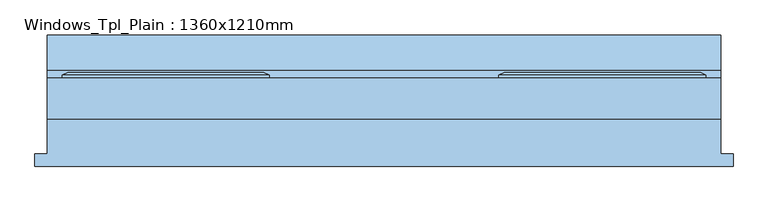
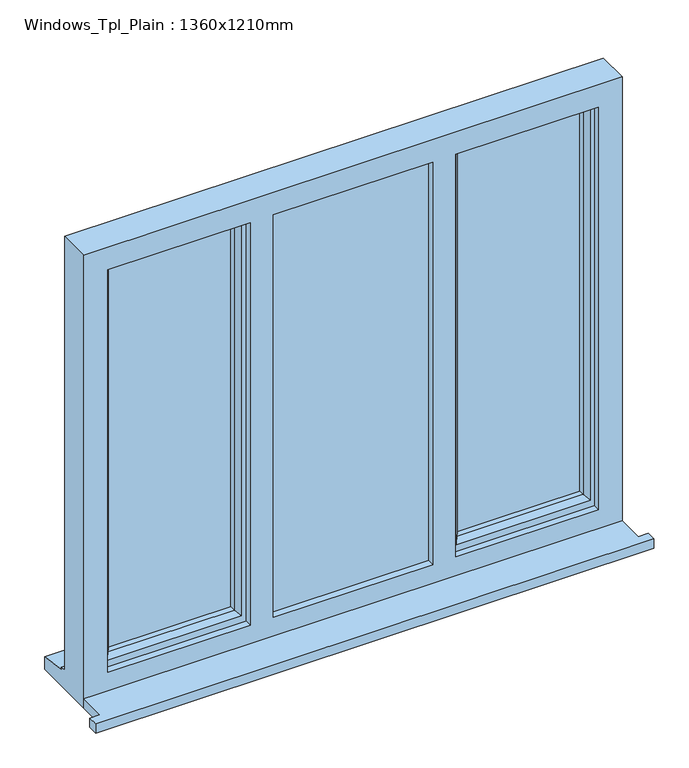
"""IFC4 building model written with IfcOpenShell, lengths in millimetres: window geometry, Windows_Tpl_Plain : 1360x1210mm."""

from ifc_helpers import new_model, si_unit, frame, origin, place, context, project, spatial, polyline, outline, extrude, faceted_brep, source, transform, mapped, element, save


def windows_tpl_plain_1360x1210mm_e2a6c9d8(model_context):
    return source(origin(), model_context, "Body", "SolidModel", [
        extrude(outline(polyline([(-1206.6666667, -118.1434322), (-1206.6666667, -93.1434322), (-1181.6666667, -93.1434322), (-1181.6666667, -22.9434322), (178.3333333, -22.9434322), (178.3333333, -93.1434322), (203.3333333, -93.1434322), (203.3333333, -118.1434322), (-1206.6666667, -118.1434322)])), frame((0.0, 0.0, 900.0), z_axis=(0.0, 0.0, 1.0), x_axis=(1.0, 0.0, 0.0)), (0.0, 0.0, 1.0), 25.0),
        faceted_brep([(-270.0, 60.0565678, 2080.0), (-270.0, 65.8300705, 2080.0), (-270.0, 65.8300705, 953.0), (-270.0, 60.0565678, 953.0), (-260.0, -4.9434322, 2070.0), (-260.0, 60.0565678, 2070.0), (-260.0, 60.0565678, 963.0), (-260.0, -4.9434322, 963.0), (-220.0, 9.5494677, 2030.0), (-230.1480377, -4.9434322, 2040.1480377), (-230.1480377, -4.9434322, 992.8519623), (-220.0, 9.5494677, 1003.0), (-220.0, 24.0565678, 2030.0), (-220.0, 24.0565678, 1003.0), (-230.0, 48.0565678, 2040.0), (-230.0, 24.0565678, 2040.0), (-230.0, 24.0565678, 993.0), (-230.0, 48.0565678, 993.0), (-220.0, 65.8300705, 2030.0), (-220.0, 48.0565678, 2030.0), (-220.0, 48.0565678, 1003.0), (-220.0, 65.8300705, 1003.0), (-237.4457548, 71.6035732, 2047.4457548), (-237.4457548, 71.6035732, 985.5542452), (-259.2153903, 71.6035732, 2069.2153903), (-259.2153903, 71.6035732, 963.7846097), (148.3333333, 65.8300705, 953.0), (148.3333333, 60.0565678, 953.0), (138.3333333, 60.0565678, 963.0), (138.3333333, -4.9434322, 963.0), (108.4813711, -4.9434322, 992.8519623), (98.3333333, 9.5494677, 1003.0), (98.3333333, 24.0565678, 1003.0), (108.3333333, 24.0565678, 993.0), (108.3333333, 48.0565678, 993.0), (98.3333333, 48.0565678, 1003.0), (98.3333333, 65.8300705, 1003.0), (115.7790881, 71.6035732, 985.5542452), (137.5487236, 71.6035732, 963.7846097), (148.3333333, 65.8300705, 2080.0), (148.3333333, 60.0565678, 2080.0), (138.3333333, 60.0565678, 2070.0), (138.3333333, -4.9434322, 2070.0), (108.4813711, -4.9434322, 2040.1480377), (98.3333333, 9.5494677, 2030.0), (98.3333333, 24.0565678, 2030.0), (108.3333333, 24.0565678, 2040.0), (108.3333333, 48.0565678, 2040.0), (98.3333333, 48.0565678, 2030.0), (98.3333333, 65.8300705, 2030.0), (115.7790881, 71.6035732, 2047.4457548), (137.5487236, 71.6035732, 2069.2153903)], [[[0, 1, 2, 3]], [[4, 5, 6, 7]], [[8, 9, 10, 11]], [[12, 8, 11, 13]], [[14, 15, 16, 17]], [[18, 19, 20, 21]], [[22, 18, 21, 23]], [[1, 24, 25, 2]], [[3, 2, 26, 27]], [[7, 6, 28, 29]], [[11, 10, 30, 31]], [[13, 11, 31, 32]], [[17, 16, 33, 34]], [[21, 20, 35, 36]], [[23, 21, 36, 37]], [[2, 25, 38, 26]], [[27, 26, 39, 40]], [[29, 28, 41, 42]], [[31, 30, 43, 44]], [[32, 31, 44, 45]], [[34, 33, 46, 47]], [[36, 35, 48, 49]], [[37, 36, 49, 50]], [[26, 38, 51, 39]], [[40, 39, 1, 0]], [[3, 27, 40, 0], [5, 41, 28, 6]], [[42, 41, 5, 4]], [[7, 29, 42, 4], [9, 43, 30, 10]], [[44, 43, 9, 8]], [[45, 44, 8, 12]], [[15, 46, 33, 16], [13, 32, 45, 12]], [[47, 46, 15, 14]], [[17, 34, 47, 14], [19, 48, 35, 20]], [[49, 48, 19, 18]], [[50, 49, 18, 22]], [[24, 51, 38, 25], [23, 37, 50, 22]], [[39, 51, 24, 1]]]),
        faceted_brep([(-733.3333333, 60.0565678, 2080.0), (-733.3333333, 65.8300705, 2080.0), (-1151.6666667, 65.8300705, 2080.0), (-1151.6666667, 60.0565678, 2080.0), (-743.3333333, -4.9434322, 2070.0), (-743.3333333, 60.0565678, 2070.0), (-1141.6666667, 60.0565678, 2070.0), (-1141.6666667, -4.9434322, 2070.0), (-783.3333333, 9.5494677, 2030.0), (-773.1852956, -4.9434322, 2040.1480377), (-1111.8147044, -4.9434322, 2040.1480377), (-1101.6666667, 9.5494677, 2030.0), (-783.3333333, 24.0565678, 2030.0), (-1101.6666667, 24.0565678, 2030.0), (-773.3333333, 48.0565678, 2040.0), (-773.3333333, 24.0565678, 2040.0), (-1111.6666667, 24.0565678, 2040.0), (-1111.6666667, 48.0565678, 2040.0), (-783.3333333, 65.8300705, 2030.0), (-783.3333333, 48.0565678, 2030.0), (-1101.6666667, 48.0565678, 2030.0), (-1101.6666667, 65.8300705, 2030.0), (-764.5187677, 71.6035732, 2048.8145656), (-1120.4812323, 71.6035732, 2048.8145656), (-744.964114, 71.6035732, 2068.3692194), (-1140.035886, 71.6035732, 2068.3692194), (-1151.6666667, 65.8300705, 953.0), (-1151.6666667, 60.0565678, 953.0), (-1141.6666667, 60.0565678, 963.0), (-1141.6666667, -4.9434322, 963.0), (-1111.8147044, -4.9434322, 992.8519623), (-1101.6666667, 9.5494677, 1003.0), (-1101.6666667, 24.0565678, 1003.0), (-1111.6666667, 24.0565678, 993.0), (-1111.6666667, 48.0565678, 993.0), (-1101.6666667, 48.0565678, 1003.0), (-1101.6666667, 65.8300705, 1003.0), (-1120.4812323, 71.6035732, 984.1854344), (-1140.035886, 71.6035732, 964.6307806), (-733.3333333, 65.8300705, 953.0), (-733.3333333, 60.0565678, 953.0), (-743.3333333, 60.0565678, 963.0), (-743.3333333, -4.9434322, 963.0), (-773.1852956, -4.9434322, 992.8519623), (-783.3333333, 9.5494677, 1003.0), (-783.3333333, 24.0565678, 1003.0), (-773.3333333, 24.0565678, 993.0), (-773.3333333, 48.0565678, 993.0), (-783.3333333, 48.0565678, 1003.0), (-783.3333333, 65.8300705, 1003.0), (-764.5187677, 71.6035732, 984.1854344), (-744.964114, 71.6035732, 964.6307806)], [[[0, 1, 2, 3]], [[4, 5, 6, 7]], [[8, 9, 10, 11]], [[12, 8, 11, 13]], [[14, 15, 16, 17]], [[18, 19, 20, 21]], [[22, 18, 21, 23]], [[1, 24, 25, 2]], [[3, 2, 26, 27]], [[7, 6, 28, 29]], [[11, 10, 30, 31]], [[13, 11, 31, 32]], [[17, 16, 33, 34]], [[21, 20, 35, 36]], [[23, 21, 36, 37]], [[2, 25, 38, 26]], [[27, 26, 39, 40]], [[0, 3, 27, 40], [41, 28, 6, 5]], [[29, 28, 41, 42]], [[4, 7, 29, 42], [43, 30, 10, 9]], [[31, 30, 43, 44]], [[32, 31, 44, 45]], [[46, 33, 16, 15], [12, 13, 32, 45]], [[34, 33, 46, 47]], [[14, 17, 34, 47], [48, 35, 20, 19]], [[36, 35, 48, 49]], [[37, 36, 49, 50]], [[51, 38, 25, 24], [22, 23, 37, 50]], [[26, 38, 51, 39]], [[40, 39, 1, 0]], [[42, 41, 5, 4]], [[44, 43, 9, 8]], [[45, 44, 8, 12]], [[47, 46, 15, 14]], [[49, 48, 19, 18]], [[50, 49, 18, 22]], [[39, 51, 24, 1]]]),
        faceted_brep([(178.3333333, -22.9434322, 2110.0), (-1181.6666667, -22.9434322, 2110.0), (-1181.6666667, -22.9434322, 900.0), (178.3333333, -22.9434322, 900.0), (118.3333333, -22.9434322, 2050.0), (118.3333333, -22.9434322, 975.0), (-242.0, -22.9434322, 975.0), (-242.0, -22.9434322, 2050.0), (-300.0, -22.9434322, 2050.0), (-300.0, -22.9434322, 975.0), (-703.3333333, -22.9434322, 975.0), (-703.3333333, -22.9434322, 2050.0), (-761.3333333, -22.9434322, 2050.0), (-761.3333333, -22.9434322, 975.0), (-1121.6666667, -22.9434322, 975.0), (-1121.6666667, -22.9434322, 2050.0), (-1181.6666667, 60.0565678, 2110.0), (-1181.6666667, 60.0565678, 951.0), (-1181.6666667, 75.0565678, 949.68767), (-1181.6666667, 75.0565678, 944.7449676), (-1181.6666667, 147.5565678, 933.8088847), (-1181.6666667, 147.5565678, 900.0), (178.3333333, 60.0565678, 2110.0), (178.3333333, 60.0565678, 951.0), (-1141.6666667, 60.0565678, 2070.0), (-1141.6666667, 60.0565678, 963.0), (-743.3333333, 60.0565678, 963.0), (-743.3333333, 60.0565678, 2070.0), (-703.3333333, 60.0565678, 2070.0), (-703.3333333, 60.0565678, 963.0), (-300.0, 60.0565678, 963.0), (-300.0, 60.0565678, 2070.0), (-260.0, 60.0565678, 2070.0), (-260.0, 60.0565678, 963.0), (138.3333333, 60.0565678, 963.0), (138.3333333, 60.0565678, 2070.0), (-1141.6666667, -4.9434322, 2070.0), (-1141.6666667, -4.9434322, 963.0), (-713.3333333, -4.9434322, 2070.0), (-290.0, -4.9434322, 2070.0), (-290.0, -4.9434322, 963.0), (-713.3333333, -4.9434322, 963.0), (-300.0, -4.9434322, 2050.0), (-703.3333333, -4.9434322, 2050.0), (-703.3333333, -4.9434322, 975.0), (-300.0, -4.9434322, 975.0), (-260.0, -4.9434322, 2070.0), (138.3333333, -4.9434322, 2070.0), (138.3333333, -4.9434322, 963.0), (-260.0, -4.9434322, 963.0), (118.3333333, -4.9434322, 2050.0), (-242.0, -4.9434322, 2050.0), (-242.0, -4.9434322, 975.0), (118.3333333, -4.9434322, 975.0), (-743.3333333, -4.9434322, 2070.0), (-743.3333333, -4.9434322, 963.0), (-761.3333333, -4.9434322, 2050.0), (-1121.6666667, -4.9434322, 2050.0), (-1121.6666667, -4.9434322, 975.0), (-761.3333333, -4.9434322, 975.0), (-703.3333333, 19.0565678, 2070.0), (-300.0, 19.0565678, 2070.0), (-290.0, 19.0565678, 2070.0), (-713.3333333, 19.0565678, 2070.0), (178.3333333, 147.5565678, 900.0), (178.3333333, 147.5565678, 933.8088847), (178.3333333, 75.0565678, 944.7449676), (178.3333333, 75.0565678, 949.68767), (-703.3333333, 19.0565678, 963.0), (-713.3333333, 19.0565678, 963.0), (-290.0, 19.0565678, 963.0), (-300.0, 19.0565678, 963.0)], [[[0, 1, 2, 3], [4, 5, 6, 7], [8, 9, 10, 11], [12, 13, 14, 15]], [[2, 1, 16, 17, 18, 19, 20, 21]], [[17, 16, 22, 23], [24, 25, 26, 27], [28, 29, 30, 31], [32, 33, 34, 35]], [[25, 24, 36, 37]], [[38, 39, 40, 41], [42, 43, 44, 45]], [[46, 47, 48, 49], [50, 51, 52, 53]], [[36, 54, 55, 37], [56, 57, 58, 59]], [[57, 15, 14, 58]], [[1, 0, 22, 16]], [[36, 24, 27, 54]], [[35, 47, 46, 32]], [[60, 28, 31, 61, 62, 39, 38, 63]], [[15, 57, 56, 12]], [[50, 4, 7, 51]], [[11, 43, 42, 8]], [[23, 22, 0, 3, 64, 65, 66, 67]], [[35, 34, 48, 47]], [[4, 50, 53, 5]], [[43, 11, 10, 44]], [[12, 56, 59, 13]], [[27, 26, 55, 54]], [[29, 28, 60, 68]], [[68, 60, 63, 69]], [[69, 63, 38, 41]], [[62, 70, 40, 39]], [[70, 62, 61, 71]], [[71, 61, 31, 30]], [[33, 32, 46, 49]], [[51, 7, 6, 52]], [[8, 42, 45, 9]], [[64, 3, 2, 21]], [[65, 64, 21, 20]], [[66, 65, 20, 19]], [[67, 66, 19, 18]], [[23, 67, 18, 17]], [[26, 25, 37, 55]], [[34, 33, 49, 48]], [[41, 40, 70, 71, 30, 29, 68, 69]], [[6, 5, 53, 52]], [[45, 44, 10, 9]], [[59, 58, 14, 13]]]),
        extrude(outline(polyline([(-773.3333333, 24.0565678), (-1111.6666667, 24.0565678), (-1111.6666667, 48.0565678), (-773.3333333, 48.0565678), (-773.3333333, 24.0565678)])), frame((0.0, 0.0, 993.0), z_axis=(0.0, 0.0, 1.0), x_axis=(1.0, 0.0, 0.0)), (0.0, 0.0, 1.0), 1047.0),
        extrude(outline(polyline([(-713.3333333, 19.0565678), (-290.0, 19.0565678), (-290.0, -4.9434322), (-713.3333333, -4.9434322), (-713.3333333, 19.0565678)])), frame((0.0, 0.0, 963.0), z_axis=(0.0, 0.0, 1.0), x_axis=(1.0, 0.0, 0.0)), (0.0, 0.0, 1.0), 1107.0),
        extrude(outline(polyline([(108.3333333, 24.0565678), (-230.0, 24.0565678), (-230.0, 48.0565678), (108.3333333, 48.0565678), (108.3333333, 24.0565678)])), frame((0.0, 0.0, 993.0), z_axis=(0.0, 0.0, 1.0), x_axis=(1.0, 0.0, 0.0)), (0.0, 0.0, 1.0), 1047.0),
    ])


if __name__ == "__main__":
    model = new_model("IFC4")
    model_context = context("Model", 3, world=origin())
    ifc_project = project(units=[si_unit("LENGTHUNIT", "METRE", prefix="MILLI")], contexts=[model_context])
    site = spatial("IfcSite", under=ifc_project)
    building = spatial("IfcBuilding", under=site)
    placement = place(None, origin())
    windows_tpl_plain_1360x1210mm_shape = windows_tpl_plain_1360x1210mm_e2a6c9d8(model_context)
    element("IfcWindow", 1, ObjectType="Windows_Tpl_Plain : 1360x1210mm", at=placement, inside=building, context=model_context, shape_type="MappedRepresentation", body=[
        mapped(windows_tpl_plain_1360x1210mm_shape, transform((0.0, 0.0, 0.0), x_axis=(1.0, 0.0, 0.0), y_axis=(0.0, 1.0, 0.0), z_axis=(0.0, 0.0, 1.0))),
    ])
    save(model, "model.ifc")

# Revit data of these elements
# Type "Windows_Tpl_Plain : 1360x1210mm"
#   Type Mark = "21"
#   Operation = "TriplePanelVertical"
#   Construction Type Id = "GSP4R"
#   Manufacturer = "Revit"
#   Keynote = "L10"
#   Analytic Construction = "1/8 in Pilkington single glazing"
#   Wrap Layers (Ext) from Ext = 0' - 4.03543"
#   Wrap Layers (Int) from Ext = 0' - 6.98819"
#   Window Board Projection = 0' - 0.98425"
#   Window Board Extension = 0' - 0.98425"
#   Visual Light Transmittance = 0.9
#   Solar Heat Gain Coefficient = 0.78
#   Rough Width = 4' - 5.54331"
#   Rough Height = 3' - 11.6378"
#   Height = 3' - 11.6378"
#   Width = 4' - 5.54331"
#   Heat Transfer Coefficient (U) = 0.6496 BTU/(h·ft²·°F)
#   Glazing Thickness = 0' - 0.94488"
#   FrameOffset - External = 0' - 1.9685"
#   Frame Depth = 0' - 2.55906"
#   Default Head Height = 6' - 11.07087"
#   Cill Depth = 0' - 3.44488"
#   Cavity Closer Width = 0' - 1.9685"
#   Cavity Closer Offset from Ext = 0' - 4.03543"
#   Cavity Closer Depth = 0' - 3.34646"
#   Vis - Cavity Closers = yes
#   Define Thermal Properties by = 1
#   Material Trim = Window Frame
#   Material Glass = Glass
#   Material Frame = Window Frame
#   Wall Closure = (empty or 0)
# Element 1 (IfcWindow, "Windows_Tpl_Plain : 1360x1210mm")
#   Materials on its faces: "Window Frame", "Glass"
# Materials
#   "Window Frame": colour RGB 249 249 249, transparency 0
#   "Glass": class "Glass", colour RGB 0 128 192, transparency 0.75, Description = "Soda Lime Glass", Cost = 0
